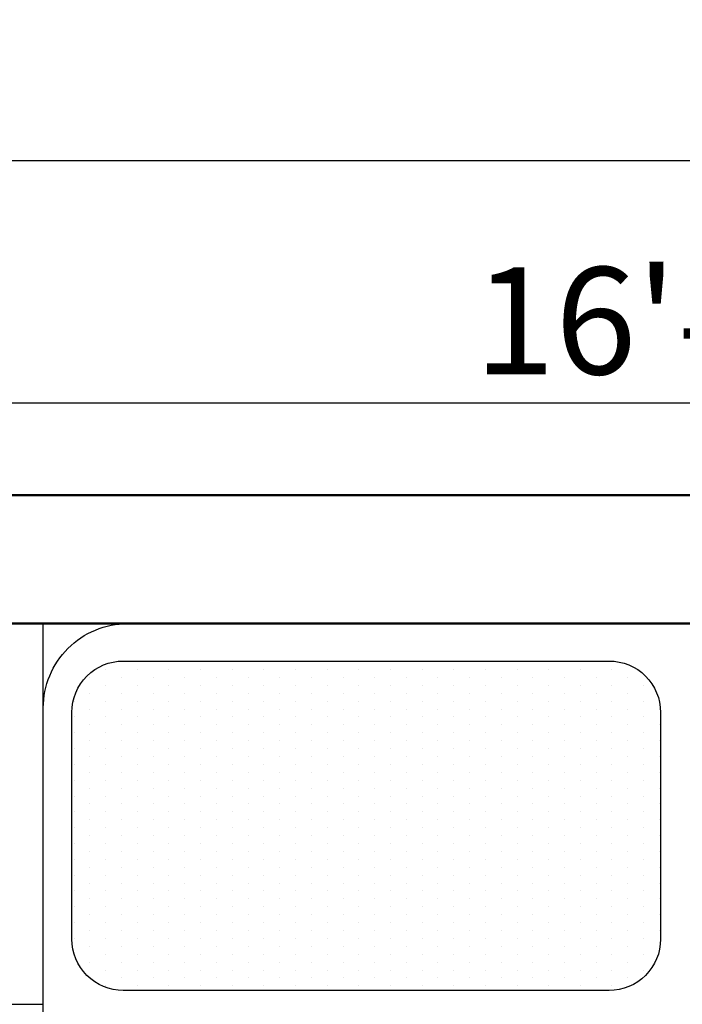
# Model space of a CAD drawing. Units: inches. Extents: x 3064 to 19385, y 846 to 15425.
# Tile 77 of 108: x 6677 to 6708, y 1964 to 2010. Entities that reach past the tile are written whole.
import ezdxf

# ---------------------------------------------------------------- set-up
doc = ezdxf.new("R2010")
doc.units = ezdxf.units.IN
for name, color, linetype, lineweight in [('A-ANNO-DIMS', 2, 'Continuous', 18), ('A-FLOR-FIXT', 9, 'Continuous', 18), ('A-WALL', 7, 'Continuous', 50)]:
    doc.layers.add(name, color=color, linetype=linetype, lineweight=lineweight)
doc.layers.add('BLOCK', color=6, linetype='Continuous')
doc.styles.get("Standard").update_dxf_attribs({"font": 'arial.ttf'})
doc.dimstyles.new('ISO-25', dxfattribs={"dimtxt": 9, "dimasz": 2.5, "dimexe": 1.25, "dimexo": 0.625, "dimtad": 1, "dimdec": 1, "dimlunit": 3, "dimtxsty": 'Standard', "dimcen": 2.5, "dimadec": 0, "dimazin": 0, "dimtfac": 1, "dimtdec": 1, "dimtmove": 0, "dimatfit": 3, "dimfxl": 1, "dimarcsym": 0})

# ---------------------------------------------------------------- blocks, each defined once
blk = doc.blocks.new('*X7')
at = {"color": 0}
for p, q in [((266.4375, 457.03125), (266.4375, 457.03125)), ((266.8125, 457.03125), (266.8125, 457.03125)), ((267.1875, 457.03125), (267.1875, 457.03125)), ((267.5625, 457.03125), (267.5625, 457.03125)), ((267.9375, 457.03125), (267.9375, 457.03125)), ((268.3125, 457.03125), (268.3125, 457.03125)), ((268.6875, 457.03125), (268.6875, 457.03125)), ((269.0625, 457.03125), (269.0625, 457.03125)), ((269.4375, 457.03125), (269.4375, 457.03125)), ((269.8125, 457.03125), (269.8125, 457.03125)), ((270.1875, 457.03125), (270.1875, 457.03125)), ((270.5625, 457.03125), (270.5625, 457.03125)), ((270.9375, 457.03125), (270.9375, 457.03125)), ((271.3125, 457.03125), (271.3125, 457.03125)), ((271.6875, 457.03125), (271.6875, 457.03125)), ((272.0625, 457.03125), (272.0625, 457.03125)), ((266.25, 456.9375), (266.25, 456.9375)), ((266.625, 456.9375), (266.625, 456.9375)), ((267, 456.9375), (267, 456.9375)), ((267.375, 456.9375), (267.375, 456.9375)), ((267.75, 456.9375), (267.75, 456.9375)), ((268.125, 456.9375), (268.125, 456.9375)), ((268.5, 456.9375), (268.5, 456.9375)), ((268.875, 456.9375), (268.875, 456.9375)), ((269.25, 456.9375), (269.25, 456.9375)), ((269.625, 456.9375), (269.625, 456.9375)), ((270, 456.9375), (270, 456.9375)), ((270.375, 456.9375), (270.375, 456.9375)), ((270.75, 456.9375), (270.75, 456.9375)), ((271.125, 456.9375), (271.125, 456.9375)), ((271.5, 456.9375), (271.5, 456.9375)), ((271.875, 456.9375), (271.875, 456.9375)), ((272.25, 456.9375), (272.25, 456.9375)), ((266.0625, 456.84375), (266.0625, 456.84375)), ((266.25, 456.75), (266.25, 456.75)), ((266.4375, 456.84375), (266.4375, 456.84375)), ((266.625, 456.75), (266.625, 456.75)), ((266.8125, 456.84375), (266.8125, 456.84375)), ((267, 456.75), (267, 456.75)), ((267.1875, 456.84375), (267.1875, 456.84375)), ((267.375, 456.75), (267.375, 456.75)), ((267.5625, 456.84375), (267.5625, 456.84375)), ((267.75, 456.75), (267.75, 456.75)), ((267.9375, 456.84375), (267.9375, 456.84375)), ((268.125, 456.75), (268.125, 456.75)), ((268.3125, 456.84375), (268.3125, 456.84375)), ((268.5, 456.75), (268.5, 456.75)), ((268.6875, 456.84375), (268.6875, 456.84375)), ((268.875, 456.75), (268.875, 456.75)), ((269.0625, 456.84375), (269.0625, 456.84375)), ((269.25, 456.75), (269.25, 456.75)), ((269.4375, 456.84375), (269.4375, 456.84375)), ((269.625, 456.75), (269.625, 456.75)), ((269.8125, 456.84375), (269.8125, 456.84375)), ((270, 456.75), (270, 456.75)), ((270.1875, 456.84375), (270.1875, 456.84375)), ((270.375, 456.75), (270.375, 456.75)), ((270.5625, 456.84375), (270.5625, 456.84375)), ((270.75, 456.75), (270.75, 456.75)), ((270.9375, 456.84375), (270.9375, 456.84375)), ((271.125, 456.75), (271.125, 456.75)), ((271.3125, 456.84375), (271.3125, 456.84375)), ((271.5, 456.75), (271.5, 456.75)), ((271.6875, 456.84375), (271.6875, 456.84375)), ((271.875, 456.75), (271.875, 456.75)), ((272.0625, 456.84375), (272.0625, 456.84375)), ((272.25, 456.75), (272.25, 456.75)), ((272.4375, 456.84375), (272.4375, 456.84375)), ((272.625, 456.75), (272.625, 456.75)), ((266.0625, 456.65625), (266.0625, 456.65625)), ((266.4375, 456.65625), (266.4375, 456.65625)), ((266.8125, 456.65625), (266.8125, 456.65625)), ((267.1875, 456.65625), (267.1875, 456.65625)), ((267.5625, 456.65625), (267.5625, 456.65625)), ((267.9375, 456.65625), (267.9375, 456.65625)), ((268.3125, 456.65625), (268.3125, 456.65625)), ((268.6875, 456.65625), (268.6875, 456.65625)), ((269.0625, 456.65625), (269.0625, 456.65625)), ((269.4375, 456.65625), (269.4375, 456.65625)), ((269.8125, 456.65625), (269.8125, 456.65625)), ((270.1875, 456.65625), (270.1875, 456.65625)), ((270.5625, 456.65625), (270.5625, 456.65625)), ((270.9375, 456.65625), (270.9375, 456.65625)), ((271.3125, 456.65625), (271.3125, 456.65625)), ((271.6875, 456.65625), (271.6875, 456.65625)), ((272.0625, 456.65625), (272.0625, 456.65625)), ((272.4375, 456.65625), (272.4375, 456.65625)), ((265.875, 456.5625), (265.875, 456.5625)), ((266.25, 456.5625), (266.25, 456.5625)), ((266.625, 456.5625), (266.625, 456.5625)), ((267, 456.5625), (267, 456.5625)), ((267.375, 456.5625), (267.375, 456.5625)), ((267.75, 456.5625), (267.75, 456.5625)), ((268.125, 456.5625), (268.125, 456.5625)), ((268.5, 456.5625), (268.5, 456.5625)), ((268.875, 456.5625), (268.875, 456.5625)), ((269.25, 456.5625), (269.25, 456.5625)), ((269.625, 456.5625), (269.625, 456.5625)), ((270, 456.5625), (270, 456.5625)), ((270.375, 456.5625), (270.375, 456.5625)), ((270.75, 456.5625), (270.75, 456.5625)), ((271.125, 456.5625), (271.125, 456.5625)), ((271.5, 456.5625), (271.5, 456.5625)), ((271.875, 456.5625), (271.875, 456.5625)), ((272.25, 456.5625), (272.25, 456.5625)), ((272.625, 456.5625), (272.625, 456.5625)), ((266.0625, 456.46875), (266.0625, 456.46875)), ((266.4375, 456.46875), (266.4375, 456.46875)), ((266.8125, 456.46875), (266.8125, 456.46875)), ((267.1875, 456.46875), (267.1875, 456.46875)), ((267.5625, 456.46875), (267.5625, 456.46875)), ((267.9375, 456.46875), (267.9375, 456.46875)), ((268.3125, 456.46875), (268.3125, 456.46875)), ((268.6875, 456.46875), (268.6875, 456.46875)), ((269.0625, 456.46875), (269.0625, 456.46875)), ((269.4375, 456.46875), (269.4375, 456.46875)), ((269.8125, 456.46875), (269.8125, 456.46875)), ((270.1875, 456.46875), (270.1875, 456.46875)), ((270.5625, 456.46875), (270.5625, 456.46875)), ((270.9375, 456.46875), (270.9375, 456.46875)), ((271.3125, 456.46875), (271.3125, 456.46875)), ((271.6875, 456.46875), (271.6875, 456.46875)), ((272.0625, 456.46875), (272.0625, 456.46875)), ((272.4375, 456.46875), (272.4375, 456.46875)), ((272.8125, 456.46875), (272.8125, 456.46875)), ((265.875, 456.375), (265.875, 456.375)), ((266.0625, 456.28125), (266.0625, 456.28125)), ((266.25, 456.375), (266.25, 456.375)), ((266.4375, 456.28125), (266.4375, 456.28125)), ((266.625, 456.375), (266.625, 456.375)), ((266.8125, 456.28125), (266.8125, 456.28125)), ((267, 456.375), (267, 456.375)), ((267.1875, 456.28125), (267.1875, 456.28125)), ((267.375, 456.375), (267.375, 456.375)), ((267.5625, 456.28125), (267.5625, 456.28125)), ((267.75, 456.375), (267.75, 456.375)), ((267.9375, 456.28125), (267.9375, 456.28125)), ((268.125, 456.375), (268.125, 456.375)), ((268.3125, 456.28125), (268.3125, 456.28125)), ((268.5, 456.375), (268.5, 456.375)), ((268.6875, 456.28125), (268.6875, 456.28125)), ((268.875, 456.375), (268.875, 456.375)), ((269.0625, 456.28125), (269.0625, 456.28125)), ((269.25, 456.375), (269.25, 456.375)), ((269.4375, 456.28125), (269.4375, 456.28125)), ((269.625, 456.375), (269.625, 456.375)), ((269.8125, 456.28125), (269.8125, 456.28125)), ((270, 456.375), (270, 456.375)), ((270.1875, 456.28125), (270.1875, 456.28125)), ((270.375, 456.375), (270.375, 456.375)), ((270.5625, 456.28125), (270.5625, 456.28125)), ((270.75, 456.375), (270.75, 456.375)), ((270.9375, 456.28125), (270.9375, 456.28125)), ((271.125, 456.375), (271.125, 456.375)), ((271.3125, 456.28125), (271.3125, 456.28125)), ((271.5, 456.375), (271.5, 456.375)), ((271.6875, 456.28125), (271.6875, 456.28125)), ((271.875, 456.375), (271.875, 456.375)), ((272.0625, 456.28125), (272.0625, 456.28125)), ((272.25, 456.375), (272.25, 456.375)), ((272.4375, 456.28125), (272.4375, 456.28125)), ((272.625, 456.375), (272.625, 456.375)), ((272.8125, 456.28125), (272.8125, 456.28125)), ((265.875, 456.1875), (265.875, 456.1875)), ((266.25, 456.1875), (266.25, 456.1875)), ((266.625, 456.1875), (266.625, 456.1875)), ((267, 456.1875), (267, 456.1875)), ((267.375, 456.1875), (267.375, 456.1875)), ((267.75, 456.1875), (267.75, 456.1875)), ((268.125, 456.1875), (268.125, 456.1875)), ((268.5, 456.1875), (268.5, 456.1875)), ((268.875, 456.1875), (268.875, 456.1875)), ((269.25, 456.1875), (269.25, 456.1875)), ((269.625, 456.1875), (269.625, 456.1875)), ((270, 456.1875), (270, 456.1875)), ((270.375, 456.1875), (270.375, 456.1875)), ((270.75, 456.1875), (270.75, 456.1875)), ((271.125, 456.1875), (271.125, 456.1875)), ((271.5, 456.1875), (271.5, 456.1875)), ((271.875, 456.1875), (271.875, 456.1875)), ((272.25, 456.1875), (272.25, 456.1875)), ((272.625, 456.1875), (272.625, 456.1875)), ((266.0625, 456.09375), (266.0625, 456.09375)), ((266.4375, 456.09375), (266.4375, 456.09375)), ((266.8125, 456.09375), (266.8125, 456.09375)), ((267.1875, 456.09375), (267.1875, 456.09375)), ((267.5625, 456.09375), (267.5625, 456.09375)), ((267.9375, 456.09375), (267.9375, 456.09375)), ((268.3125, 456.09375), (268.3125, 456.09375)), ((268.6875, 456.09375), (268.6875, 456.09375)), ((269.0625, 456.09375), (269.0625, 456.09375)), ((269.4375, 456.09375), (269.4375, 456.09375)), ((269.8125, 456.09375), (269.8125, 456.09375)), ((270.1875, 456.09375), (270.1875, 456.09375)), ((270.5625, 456.09375), (270.5625, 456.09375)), ((270.9375, 456.09375), (270.9375, 456.09375)), ((271.3125, 456.09375), (271.3125, 456.09375)), ((271.6875, 456.09375), (271.6875, 456.09375)), ((272.0625, 456.09375), (272.0625, 456.09375)), ((272.4375, 456.09375), (272.4375, 456.09375)), ((272.8125, 456.09375), (272.8125, 456.09375)), ((265.875, 456), (265.875, 456)), ((266.25, 456), (266.25, 456)), ((266.625, 456), (266.625, 456)), ((267, 456), (267, 456)), ((267.375, 456), (267.375, 456)), ((267.75, 456), (267.75, 456)), ((268.125, 456), (268.125, 456)), ((268.5, 456), (268.5, 456)), ((268.875, 456), (268.875, 456)), ((269.25, 456), (269.25, 456)), ((269.625, 456), (269.625, 456)), ((270, 456), (270, 456)), ((270.375, 456), (270.375, 456)), ((270.75, 456), (270.75, 456)), ((271.125, 456), (271.125, 456)), ((271.5, 456), (271.5, 456)), ((271.875, 456), (271.875, 456)), ((272.25, 456), (272.25, 456)), ((272.625, 456), (272.625, 456)), ((265.875, 455.8125), (265.875, 455.8125)), ((266.0625, 455.90625), (266.0625, 455.90625)), ((266.25, 455.8125), (266.25, 455.8125)), ((266.4375, 455.90625), (266.4375, 455.90625)), ((266.625, 455.8125), (266.625, 455.8125)), ((266.8125, 455.90625), (266.8125, 455.90625)), ((267, 455.8125), (267, 455.8125)), ((267.1875, 455.90625), (267.1875, 455.90625)), ((267.375, 455.8125), (267.375, 455.8125)), ((267.5625, 455.90625), (267.5625, 455.90625)), ((267.75, 455.8125), (267.75, 455.8125)), ((267.9375, 455.90625), (267.9375, 455.90625)), ((268.125, 455.8125), (268.125, 455.8125)), ((268.3125, 455.90625), (268.3125, 455.90625)), ((268.5, 455.8125), (268.5, 455.8125)), ((268.6875, 455.90625), (268.6875, 455.90625)), ((268.875, 455.8125), (268.875, 455.8125)), ((269.0625, 455.90625), (269.0625, 455.90625)), ((269.25, 455.8125), (269.25, 455.8125)), ((269.4375, 455.90625), (269.4375, 455.90625)), ((269.625, 455.8125), (269.625, 455.8125)), ((269.8125, 455.90625), (269.8125, 455.90625)), ((270, 455.8125), (270, 455.8125)), ((270.1875, 455.90625), (270.1875, 455.90625)), ((270.375, 455.8125), (270.375, 455.8125)), ((270.5625, 455.90625), (270.5625, 455.90625)), ((270.75, 455.8125), (270.75, 455.8125)), ((270.9375, 455.90625), (270.9375, 455.90625)), ((271.125, 455.8125), (271.125, 455.8125)), ((271.3125, 455.90625), (271.3125, 455.90625)), ((271.5, 455.8125), (271.5, 455.8125)), ((271.6875, 455.90625), (271.6875, 455.90625)), ((271.875, 455.8125), (271.875, 455.8125)), ((272.0625, 455.90625), (272.0625, 455.90625)), ((272.25, 455.8125), (272.25, 455.8125)), ((272.4375, 455.90625), (272.4375, 455.90625)), ((272.625, 455.8125), (272.625, 455.8125)), ((272.8125, 455.90625), (272.8125, 455.90625)), ((266.0625, 455.71875), (266.0625, 455.71875)), ((266.4375, 455.71875), (266.4375, 455.71875)), ((266.8125, 455.71875), (266.8125, 455.71875)), ((267.1875, 455.71875), (267.1875, 455.71875)), ((267.5625, 455.71875), (267.5625, 455.71875)), ((267.9375, 455.71875), (267.9375, 455.71875)), ((268.3125, 455.71875), (268.3125, 455.71875)), ((268.6875, 455.71875), (268.6875, 455.71875)), ((269.0625, 455.71875), (269.0625, 455.71875)), ((269.4375, 455.71875), (269.4375, 455.71875)), ((269.8125, 455.71875), (269.8125, 455.71875)), ((270.1875, 455.71875), (270.1875, 455.71875)), ((270.5625, 455.71875), (270.5625, 455.71875)), ((270.9375, 455.71875), (270.9375, 455.71875)), ((271.3125, 455.71875), (271.3125, 455.71875)), ((271.6875, 455.71875), (271.6875, 455.71875)), ((272.0625, 455.71875), (272.0625, 455.71875)), ((272.4375, 455.71875), (272.4375, 455.71875)), ((272.8125, 455.71875), (272.8125, 455.71875)), ((265.875, 455.625), (265.875, 455.625)), ((266.25, 455.625), (266.25, 455.625)), ((266.625, 455.625), (266.625, 455.625)), ((267, 455.625), (267, 455.625)), ((267.375, 455.625), (267.375, 455.625)), ((267.75, 455.625), (267.75, 455.625)), ((268.125, 455.625), (268.125, 455.625)), ((268.5, 455.625), (268.5, 455.625)), ((268.875, 455.625), (268.875, 455.625)), ((269.25, 455.625), (269.25, 455.625)), ((269.625, 455.625), (269.625, 455.625)), ((270, 455.625), (270, 455.625)), ((270.375, 455.625), (270.375, 455.625)), ((270.75, 455.625), (270.75, 455.625)), ((271.125, 455.625), (271.125, 455.625)), ((271.5, 455.625), (271.5, 455.625)), ((271.875, 455.625), (271.875, 455.625)), ((272.25, 455.625), (272.25, 455.625)), ((272.625, 455.625), (272.625, 455.625)), ((266.0625, 455.53125), (266.0625, 455.53125)), ((266.4375, 455.53125), (266.4375, 455.53125)), ((266.8125, 455.53125), (266.8125, 455.53125)), ((267.1875, 455.53125), (267.1875, 455.53125)), ((267.5625, 455.53125), (267.5625, 455.53125)), ((267.9375, 455.53125), (267.9375, 455.53125)), ((268.3125, 455.53125), (268.3125, 455.53125)), ((268.6875, 455.53125), (268.6875, 455.53125)), ((269.0625, 455.53125), (269.0625, 455.53125)), ((269.4375, 455.53125), (269.4375, 455.53125)), ((269.8125, 455.53125), (269.8125, 455.53125)), ((270.1875, 455.53125), (270.1875, 455.53125)), ((270.5625, 455.53125), (270.5625, 455.53125)), ((270.9375, 455.53125), (270.9375, 455.53125)), ((271.3125, 455.53125), (271.3125, 455.53125)), ((271.6875, 455.53125), (271.6875, 455.53125)), ((272.0625, 455.53125), (272.0625, 455.53125)), ((272.4375, 455.53125), (272.4375, 455.53125)), ((272.8125, 455.53125), (272.8125, 455.53125)), ((265.875, 455.4375), (265.875, 455.4375)), ((266.0625, 455.34375), (266.0625, 455.34375)), ((266.25, 455.4375), (266.25, 455.4375)), ((266.4375, 455.34375), (266.4375, 455.34375)), ((266.625, 455.4375), (266.625, 455.4375)), ((266.8125, 455.34375), (266.8125, 455.34375)), ((267, 455.4375), (267, 455.4375)), ((267.1875, 455.34375), (267.1875, 455.34375)), ((267.375, 455.4375), (267.375, 455.4375)), ((267.5625, 455.34375), (267.5625, 455.34375)), ((267.75, 455.4375), (267.75, 455.4375)), ((267.9375, 455.34375), (267.9375, 455.34375)), ((268.125, 455.4375), (268.125, 455.4375)), ((268.3125, 455.34375), (268.3125, 455.34375)), ((268.5, 455.4375), (268.5, 455.4375)), ((268.6875, 455.34375), (268.6875, 455.34375)), ((268.875, 455.4375), (268.875, 455.4375)), ((269.0625, 455.34375), (269.0625, 455.34375)), ((269.25, 455.4375), (269.25, 455.4375)), ((269.4375, 455.34375), (269.4375, 455.34375)), ((269.625, 455.4375), (269.625, 455.4375)), ((269.8125, 455.34375), (269.8125, 455.34375)), ((270, 455.4375), (270, 455.4375)), ((270.1875, 455.34375), (270.1875, 455.34375)), ((270.375, 455.4375), (270.375, 455.4375)), ((270.5625, 455.34375), (270.5625, 455.34375)), ((270.75, 455.4375), (270.75, 455.4375)), ((270.9375, 455.34375), (270.9375, 455.34375)), ((271.125, 455.4375), (271.125, 455.4375)), ((271.3125, 455.34375), (271.3125, 455.34375)), ((271.5, 455.4375), (271.5, 455.4375)), ((271.6875, 455.34375), (271.6875, 455.34375)), ((271.875, 455.4375), (271.875, 455.4375)), ((272.0625, 455.34375), (272.0625, 455.34375)), ((272.25, 455.4375), (272.25, 455.4375)), ((272.4375, 455.34375), (272.4375, 455.34375)), ((272.625, 455.4375), (272.625, 455.4375)), ((272.8125, 455.34375), (272.8125, 455.34375)), ((265.875, 455.25), (265.875, 455.25)), ((266.25, 455.25), (266.25, 455.25)), ((266.625, 455.25), (266.625, 455.25)), ((267, 455.25), (267, 455.25)), ((267.375, 455.25), (267.375, 455.25)), ((267.75, 455.25), (267.75, 455.25)), ((268.125, 455.25), (268.125, 455.25)), ((268.5, 455.25), (268.5, 455.25)), ((268.875, 455.25), (268.875, 455.25)), ((269.25, 455.25), (269.25, 455.25)), ((269.625, 455.25), (269.625, 455.25)), ((270, 455.25), (270, 455.25)), ((270.375, 455.25), (270.375, 455.25)), ((270.75, 455.25), (270.75, 455.25)), ((271.125, 455.25), (271.125, 455.25)), ((271.5, 455.25), (271.5, 455.25)), ((271.875, 455.25), (271.875, 455.25)), ((272.25, 455.25), (272.25, 455.25)), ((272.625, 455.25), (272.625, 455.25)), ((266.0625, 455.15625), (266.0625, 455.15625)), ((266.4375, 455.15625), (266.4375, 455.15625)), ((266.8125, 455.15625), (266.8125, 455.15625)), ((267.1875, 455.15625), (267.1875, 455.15625)), ((267.5625, 455.15625), (267.5625, 455.15625)), ((267.9375, 455.15625), (267.9375, 455.15625)), ((268.3125, 455.15625), (268.3125, 455.15625)), ((268.6875, 455.15625), (268.6875, 455.15625)), ((269.0625, 455.15625), (269.0625, 455.15625)), ((269.4375, 455.15625), (269.4375, 455.15625)), ((269.8125, 455.15625), (269.8125, 455.15625)), ((270.1875, 455.15625), (270.1875, 455.15625)), ((270.5625, 455.15625), (270.5625, 455.15625)), ((270.9375, 455.15625), (270.9375, 455.15625)), ((271.3125, 455.15625), (271.3125, 455.15625)), ((271.6875, 455.15625), (271.6875, 455.15625)), ((272.0625, 455.15625), (272.0625, 455.15625)), ((272.4375, 455.15625), (272.4375, 455.15625)), ((272.8125, 455.15625), (272.8125, 455.15625)), ((265.875, 455.0625), (265.875, 455.0625)), ((266.25, 455.0625), (266.25, 455.0625)), ((266.625, 455.0625), (266.625, 455.0625)), ((267, 455.0625), (267, 455.0625)), ((267.375, 455.0625), (267.375, 455.0625)), ((267.75, 455.0625), (267.75, 455.0625)), ((268.125, 455.0625), (268.125, 455.0625)), ((268.5, 455.0625), (268.5, 455.0625)), ((268.875, 455.0625), (268.875, 455.0625)), ((269.25, 455.0625), (269.25, 455.0625)), ((269.625, 455.0625), (269.625, 455.0625)), ((270, 455.0625), (270, 455.0625)), ((270.375, 455.0625), (270.375, 455.0625)), ((270.75, 455.0625), (270.75, 455.0625)), ((271.125, 455.0625), (271.125, 455.0625)), ((271.5, 455.0625), (271.5, 455.0625)), ((271.875, 455.0625), (271.875, 455.0625)), ((272.25, 455.0625), (272.25, 455.0625)), ((272.625, 455.0625), (272.625, 455.0625)), ((265.875, 454.875), (265.875, 454.875)), ((266.0625, 454.96875), (266.0625, 454.96875)), ((266.25, 454.875), (266.25, 454.875)), ((266.4375, 454.96875), (266.4375, 454.96875)), ((266.625, 454.875), (266.625, 454.875)), ((266.8125, 454.96875), (266.8125, 454.96875)), ((267, 454.875), (267, 454.875)), ((267.1875, 454.96875), (267.1875, 454.96875)), ((267.375, 454.875), (267.375, 454.875)), ((267.5625, 454.96875), (267.5625, 454.96875)), ((267.75, 454.875), (267.75, 454.875)), ((267.9375, 454.96875), (267.9375, 454.96875)), ((268.125, 454.875), (268.125, 454.875)), ((268.3125, 454.96875), (268.3125, 454.96875)), ((268.5, 454.875), (268.5, 454.875)), ((268.6875, 454.96875), (268.6875, 454.96875)), ((268.875, 454.875), (268.875, 454.875)), ((269.0625, 454.96875), (269.0625, 454.96875)), ((269.25, 454.875), (269.25, 454.875)), ((269.4375, 454.96875), (269.4375, 454.96875)), ((269.625, 454.875), (269.625, 454.875)), ((269.8125, 454.96875), (269.8125, 454.96875)), ((270, 454.875), (270, 454.875)), ((270.1875, 454.96875), (270.1875, 454.96875)), ((270.375, 454.875), (270.375, 454.875)), ((270.5625, 454.96875), (270.5625, 454.96875)), ((270.75, 454.875), (270.75, 454.875)), ((270.9375, 454.96875), (270.9375, 454.96875)), ((271.125, 454.875), (271.125, 454.875)), ((271.3125, 454.96875), (271.3125, 454.96875)), ((271.5, 454.875), (271.5, 454.875)), ((271.6875, 454.96875), (271.6875, 454.96875)), ((271.875, 454.875), (271.875, 454.875)), ((272.0625, 454.96875), (272.0625, 454.96875)), ((272.25, 454.875), (272.25, 454.875)), ((272.4375, 454.96875), (272.4375, 454.96875)), ((272.625, 454.875), (272.625, 454.875)), ((272.8125, 454.96875), (272.8125, 454.96875)), ((266.0625, 454.78125), (266.0625, 454.78125)), ((266.4375, 454.78125), (266.4375, 454.78125)), ((266.8125, 454.78125), (266.8125, 454.78125)), ((267.1875, 454.78125), (267.1875, 454.78125)), ((267.5625, 454.78125), (267.5625, 454.78125)), ((267.9375, 454.78125), (267.9375, 454.78125)), ((268.3125, 454.78125), (268.3125, 454.78125)), ((268.6875, 454.78125), (268.6875, 454.78125)), ((269.0625, 454.78125), (269.0625, 454.78125)), ((269.4375, 454.78125), (269.4375, 454.78125)), ((269.8125, 454.78125), (269.8125, 454.78125)), ((270.1875, 454.78125), (270.1875, 454.78125)), ((270.5625, 454.78125), (270.5625, 454.78125)), ((270.9375, 454.78125), (270.9375, 454.78125)), ((271.3125, 454.78125), (271.3125, 454.78125)), ((271.6875, 454.78125), (271.6875, 454.78125)), ((272.0625, 454.78125), (272.0625, 454.78125)), ((272.4375, 454.78125), (272.4375, 454.78125)), ((272.8125, 454.78125), (272.8125, 454.78125)), ((265.875, 454.6875), (265.875, 454.6875)), ((266.25, 454.6875), (266.25, 454.6875)), ((266.625, 454.6875), (266.625, 454.6875)), ((267, 454.6875), (267, 454.6875)), ((267.375, 454.6875), (267.375, 454.6875)), ((267.75, 454.6875), (267.75, 454.6875)), ((268.125, 454.6875), (268.125, 454.6875)), ((268.5, 454.6875), (268.5, 454.6875)), ((268.875, 454.6875), (268.875, 454.6875)), ((269.25, 454.6875), (269.25, 454.6875)), ((269.625, 454.6875), (269.625, 454.6875)), ((270, 454.6875), (270, 454.6875)), ((270.375, 454.6875), (270.375, 454.6875)), ((270.75, 454.6875), (270.75, 454.6875)), ((271.125, 454.6875), (271.125, 454.6875)), ((271.5, 454.6875), (271.5, 454.6875)), ((271.875, 454.6875), (271.875, 454.6875)), ((272.25, 454.6875), (272.25, 454.6875)), ((272.625, 454.6875), (272.625, 454.6875)), ((266.0625, 454.59375), (266.0625, 454.59375)), ((266.4375, 454.59375), (266.4375, 454.59375)), ((266.8125, 454.59375), (266.8125, 454.59375)), ((267.1875, 454.59375), (267.1875, 454.59375)), ((267.5625, 454.59375), (267.5625, 454.59375)), ((267.9375, 454.59375), (267.9375, 454.59375)), ((268.3125, 454.59375), (268.3125, 454.59375)), ((268.6875, 454.59375), (268.6875, 454.59375)), ((269.0625, 454.59375), (269.0625, 454.59375)), ((269.4375, 454.59375), (269.4375, 454.59375)), ((269.8125, 454.59375), (269.8125, 454.59375)), ((270.1875, 454.59375), (270.1875, 454.59375)), ((270.5625, 454.59375), (270.5625, 454.59375)), ((270.9375, 454.59375), (270.9375, 454.59375)), ((271.3125, 454.59375), (271.3125, 454.59375)), ((271.6875, 454.59375), (271.6875, 454.59375)), ((272.0625, 454.59375), (272.0625, 454.59375)), ((272.4375, 454.59375), (272.4375, 454.59375)), ((272.8125, 454.59375), (272.8125, 454.59375)), ((265.875, 454.5), (265.875, 454.5)), ((266.0625, 454.40625), (266.0625, 454.40625)), ((266.25, 454.5), (266.25, 454.5)), ((266.4375, 454.40625), (266.4375, 454.40625)), ((266.625, 454.5), (266.625, 454.5)), ((266.8125, 454.40625), (266.8125, 454.40625)), ((267, 454.5), (267, 454.5)), ((267.1875, 454.40625), (267.1875, 454.40625)), ((267.375, 454.5), (267.375, 454.5)), ((267.5625, 454.40625), (267.5625, 454.40625)), ((267.75, 454.5), (267.75, 454.5)), ((267.9375, 454.40625), (267.9375, 454.40625)), ((268.125, 454.5), (268.125, 454.5)), ((268.3125, 454.40625), (268.3125, 454.40625)), ((268.5, 454.5), (268.5, 454.5)), ((268.6875, 454.40625), (268.6875, 454.40625)), ((268.875, 454.5), (268.875, 454.5)), ((269.0625, 454.40625), (269.0625, 454.40625)), ((269.25, 454.5), (269.25, 454.5)), ((269.4375, 454.40625), (269.4375, 454.40625)), ((269.625, 454.5), (269.625, 454.5)), ((269.8125, 454.40625), (269.8125, 454.40625)), ((270, 454.5), (270, 454.5)), ((270.1875, 454.40625), (270.1875, 454.40625)), ((270.375, 454.5), (270.375, 454.5)), ((270.5625, 454.40625), (270.5625, 454.40625)), ((270.75, 454.5), (270.75, 454.5)), ((270.9375, 454.40625), (270.9375, 454.40625)), ((271.125, 454.5), (271.125, 454.5)), ((271.3125, 454.40625), (271.3125, 454.40625)), ((271.5, 454.5), (271.5, 454.5)), ((271.6875, 454.40625), (271.6875, 454.40625)), ((271.875, 454.5), (271.875, 454.5)), ((272.0625, 454.40625), (272.0625, 454.40625)), ((272.25, 454.5), (272.25, 454.5)), ((272.4375, 454.40625), (272.4375, 454.40625)), ((272.625, 454.5), (272.625, 454.5)), ((272.8125, 454.40625), (272.8125, 454.40625)), ((265.875, 454.3125), (265.875, 454.3125)), ((266.25, 454.3125), (266.25, 454.3125)), ((266.625, 454.3125), (266.625, 454.3125)), ((267, 454.3125), (267, 454.3125)), ((267.375, 454.3125), (267.375, 454.3125)), ((267.75, 454.3125), (267.75, 454.3125)), ((268.125, 454.3125), (268.125, 454.3125)), ((268.5, 454.3125), (268.5, 454.3125)), ((268.875, 454.3125), (268.875, 454.3125)), ((269.25, 454.3125), (269.25, 454.3125)), ((269.625, 454.3125), (269.625, 454.3125)), ((270, 454.3125), (270, 454.3125)), ((270.375, 454.3125), (270.375, 454.3125)), ((270.75, 454.3125), (270.75, 454.3125)), ((271.125, 454.3125), (271.125, 454.3125)), ((271.5, 454.3125), (271.5, 454.3125)), ((271.875, 454.3125), (271.875, 454.3125)), ((272.25, 454.3125), (272.25, 454.3125)), ((272.625, 454.3125), (272.625, 454.3125)), ((266.0625, 454.21875), (266.0625, 454.21875)), ((266.4375, 454.21875), (266.4375, 454.21875)), ((266.8125, 454.21875), (266.8125, 454.21875)), ((267.1875, 454.21875), (267.1875, 454.21875)), ((267.5625, 454.21875), (267.5625, 454.21875)), ((267.9375, 454.21875), (267.9375, 454.21875)), ((268.3125, 454.21875), (268.3125, 454.21875)), ((268.6875, 454.21875), (268.6875, 454.21875)), ((269.0625, 454.21875), (269.0625, 454.21875)), ((269.4375, 454.21875), (269.4375, 454.21875)), ((269.8125, 454.21875), (269.8125, 454.21875)), ((270.1875, 454.21875), (270.1875, 454.21875)), ((270.5625, 454.21875), (270.5625, 454.21875)), ((270.9375, 454.21875), (270.9375, 454.21875)), ((271.3125, 454.21875), (271.3125, 454.21875)), ((271.6875, 454.21875), (271.6875, 454.21875)), ((272.0625, 454.21875), (272.0625, 454.21875)), ((272.4375, 454.21875), (272.4375, 454.21875)), ((272.8125, 454.21875), (272.8125, 454.21875)), ((265.875, 454.125), (265.875, 454.125)), ((266.25, 454.125), (266.25, 454.125)), ((266.625, 454.125), (266.625, 454.125)), ((267, 454.125), (267, 454.125)), ((267.375, 454.125), (267.375, 454.125)), ((267.75, 454.125), (267.75, 454.125)), ((268.125, 454.125), (268.125, 454.125)), ((268.5, 454.125), (268.5, 454.125)), ((268.875, 454.125), (268.875, 454.125)), ((269.25, 454.125), (269.25, 454.125)), ((269.625, 454.125), (269.625, 454.125)), ((270, 454.125), (270, 454.125)), ((270.375, 454.125), (270.375, 454.125)), ((270.75, 454.125), (270.75, 454.125)), ((271.125, 454.125), (271.125, 454.125)), ((271.5, 454.125), (271.5, 454.125)), ((271.875, 454.125), (271.875, 454.125)), ((272.25, 454.125), (272.25, 454.125)), ((272.625, 454.125), (272.625, 454.125)), ((265.875, 453.9375), (265.875, 453.9375)), ((266.0625, 454.03125), (266.0625, 454.03125)), ((266.25, 453.9375), (266.25, 453.9375)), ((266.4375, 454.03125), (266.4375, 454.03125)), ((266.625, 453.9375), (266.625, 453.9375)), ((266.8125, 454.03125), (266.8125, 454.03125)), ((267, 453.9375), (267, 453.9375)), ((267.1875, 454.03125), (267.1875, 454.03125)), ((267.375, 453.9375), (267.375, 453.9375)), ((267.5625, 454.03125), (267.5625, 454.03125)), ((267.75, 453.9375), (267.75, 453.9375)), ((267.9375, 454.03125), (267.9375, 454.03125)), ((268.125, 453.9375), (268.125, 453.9375)), ((268.3125, 454.03125), (268.3125, 454.03125)), ((268.5, 453.9375), (268.5, 453.9375)), ((268.6875, 454.03125), (268.6875, 454.03125)), ((268.875, 453.9375), (268.875, 453.9375)), ((269.0625, 454.03125), (269.0625, 454.03125)), ((269.25, 453.9375), (269.25, 453.9375)), ((269.4375, 454.03125), (269.4375, 454.03125)), ((269.625, 453.9375), (269.625, 453.9375)), ((269.8125, 454.03125), (269.8125, 454.03125)), ((270, 453.9375), (270, 453.9375)), ((270.1875, 454.03125), (270.1875, 454.03125)), ((270.375, 453.9375), (270.375, 453.9375)), ((270.5625, 454.03125), (270.5625, 454.03125)), ((270.75, 453.9375), (270.75, 453.9375)), ((270.9375, 454.03125), (270.9375, 454.03125)), ((271.125, 453.9375), (271.125, 453.9375)), ((271.3125, 454.03125), (271.3125, 454.03125)), ((271.5, 453.9375), (271.5, 453.9375)), ((271.6875, 454.03125), (271.6875, 454.03125)), ((271.875, 453.9375), (271.875, 453.9375)), ((272.0625, 454.03125), (272.0625, 454.03125)), ((272.25, 453.9375), (272.25, 453.9375)), ((272.4375, 454.03125), (272.4375, 454.03125)), ((272.625, 453.9375), (272.625, 453.9375)), ((272.8125, 454.03125), (272.8125, 454.03125)), ((266.0625, 453.84375), (266.0625, 453.84375)), ((266.4375, 453.84375), (266.4375, 453.84375)), ((266.8125, 453.84375), (266.8125, 453.84375)), ((267.1875, 453.84375), (267.1875, 453.84375)), ((267.5625, 453.84375), (267.5625, 453.84375)), ((267.9375, 453.84375), (267.9375, 453.84375)), ((268.3125, 453.84375), (268.3125, 453.84375)), ((268.6875, 453.84375), (268.6875, 453.84375)), ((269.0625, 453.84375), (269.0625, 453.84375)), ((269.4375, 453.84375), (269.4375, 453.84375)), ((269.8125, 453.84375), (269.8125, 453.84375)), ((270.1875, 453.84375), (270.1875, 453.84375)), ((270.5625, 453.84375), (270.5625, 453.84375)), ((270.9375, 453.84375), (270.9375, 453.84375)), ((271.3125, 453.84375), (271.3125, 453.84375)), ((271.6875, 453.84375), (271.6875, 453.84375)), ((272.0625, 453.84375), (272.0625, 453.84375)), ((272.4375, 453.84375), (272.4375, 453.84375)), ((272.8125, 453.84375), (272.8125, 453.84375)), ((265.875, 453.75), (265.875, 453.75)), ((266.25, 453.75), (266.25, 453.75)), ((266.625, 453.75), (266.625, 453.75)), ((267, 453.75), (267, 453.75)), ((267.375, 453.75), (267.375, 453.75)), ((267.75, 453.75), (267.75, 453.75)), ((268.125, 453.75), (268.125, 453.75)), ((268.5, 453.75), (268.5, 453.75)), ((268.875, 453.75), (268.875, 453.75)), ((269.25, 453.75), (269.25, 453.75)), ((269.625, 453.75), (269.625, 453.75)), ((270, 453.75), (270, 453.75)), ((270.375, 453.75), (270.375, 453.75)), ((270.75, 453.75), (270.75, 453.75)), ((271.125, 453.75), (271.125, 453.75)), ((271.5, 453.75), (271.5, 453.75)), ((271.875, 453.75), (271.875, 453.75)), ((272.25, 453.75), (272.25, 453.75)), ((272.625, 453.75), (272.625, 453.75)), ((266.0625, 453.65625), (266.0625, 453.65625)), ((266.4375, 453.65625), (266.4375, 453.65625)), ((266.8125, 453.65625), (266.8125, 453.65625)), ((267.1875, 453.65625), (267.1875, 453.65625)), ((267.5625, 453.65625), (267.5625, 453.65625)), ((267.9375, 453.65625), (267.9375, 453.65625)), ((268.3125, 453.65625), (268.3125, 453.65625)), ((268.6875, 453.65625), (268.6875, 453.65625)), ((269.0625, 453.65625), (269.0625, 453.65625)), ((269.4375, 453.65625), (269.4375, 453.65625)), ((269.8125, 453.65625), (269.8125, 453.65625)), ((270.1875, 453.65625), (270.1875, 453.65625)), ((270.5625, 453.65625), (270.5625, 453.65625)), ((270.9375, 453.65625), (270.9375, 453.65625)), ((271.3125, 453.65625), (271.3125, 453.65625)), ((271.6875, 453.65625), (271.6875, 453.65625)), ((272.0625, 453.65625), (272.0625, 453.65625)), ((272.4375, 453.65625), (272.4375, 453.65625)), ((272.8125, 453.65625), (272.8125, 453.65625)), ((266.0625, 453.46875), (266.0625, 453.46875)), ((266.25, 453.5625), (266.25, 453.5625)), ((266.4375, 453.46875), (266.4375, 453.46875)), ((266.625, 453.5625), (266.625, 453.5625)), ((266.8125, 453.46875), (266.8125, 453.46875)), ((267, 453.5625), (267, 453.5625)), ((267.1875, 453.46875), (267.1875, 453.46875)), ((267.375, 453.5625), (267.375, 453.5625)), ((267.5625, 453.46875), (267.5625, 453.46875)), ((267.75, 453.5625), (267.75, 453.5625)), ((267.9375, 453.46875), (267.9375, 453.46875)), ((268.125, 453.5625), (268.125, 453.5625)), ((268.3125, 453.46875), (268.3125, 453.46875)), ((268.5, 453.5625), (268.5, 453.5625)), ((268.6875, 453.46875), (268.6875, 453.46875)), ((268.875, 453.5625), (268.875, 453.5625)), ((269.0625, 453.46875), (269.0625, 453.46875)), ((269.25, 453.5625), (269.25, 453.5625)), ((269.4375, 453.46875), (269.4375, 453.46875)), ((269.625, 453.5625), (269.625, 453.5625)), ((269.8125, 453.46875), (269.8125, 453.46875)), ((270, 453.5625), (270, 453.5625)), ((270.1875, 453.46875), (270.1875, 453.46875)), ((270.375, 453.5625), (270.375, 453.5625)), ((270.5625, 453.46875), (270.5625, 453.46875)), ((270.75, 453.5625), (270.75, 453.5625)), ((270.9375, 453.46875), (270.9375, 453.46875)), ((271.125, 453.5625), (271.125, 453.5625)), ((271.3125, 453.46875), (271.3125, 453.46875)), ((271.5, 453.5625), (271.5, 453.5625)), ((271.6875, 453.46875), (271.6875, 453.46875)), ((271.875, 453.5625), (271.875, 453.5625)), ((272.0625, 453.46875), (272.0625, 453.46875)), ((272.25, 453.5625), (272.25, 453.5625)), ((272.4375, 453.46875), (272.4375, 453.46875)), ((272.625, 453.5625), (272.625, 453.5625)), ((266.25, 453.375), (266.25, 453.375)), ((266.625, 453.375), (266.625, 453.375)), ((267, 453.375), (267, 453.375)), ((267.375, 453.375), (267.375, 453.375)), ((267.75, 453.375), (267.75, 453.375)), ((268.125, 453.375), (268.125, 453.375)), ((268.5, 453.375), (268.5, 453.375)), ((268.875, 453.375), (268.875, 453.375)), ((269.25, 453.375), (269.25, 453.375)), ((269.625, 453.375), (269.625, 453.375)), ((270, 453.375), (270, 453.375)), ((270.375, 453.375), (270.375, 453.375)), ((270.75, 453.375), (270.75, 453.375)), ((271.125, 453.375), (271.125, 453.375)), ((271.5, 453.375), (271.5, 453.375)), ((271.875, 453.375), (271.875, 453.375)), ((272.25, 453.375), (272.25, 453.375)), ((272.625, 453.375), (272.625, 453.375)), ((266.0625, 453.28125), (266.0625, 453.28125)), ((266.4375, 453.28125), (266.4375, 453.28125)), ((266.8125, 453.28125), (266.8125, 453.28125)), ((267.1875, 453.28125), (267.1875, 453.28125)), ((267.5625, 453.28125), (267.5625, 453.28125)), ((267.9375, 453.28125), (267.9375, 453.28125)), ((268.3125, 453.28125), (268.3125, 453.28125)), ((268.6875, 453.28125), (268.6875, 453.28125)), ((269.0625, 453.28125), (269.0625, 453.28125)), ((269.4375, 453.28125), (269.4375, 453.28125)), ((269.8125, 453.28125), (269.8125, 453.28125)), ((270.1875, 453.28125), (270.1875, 453.28125)), ((270.5625, 453.28125), (270.5625, 453.28125)), ((270.9375, 453.28125), (270.9375, 453.28125)), ((271.3125, 453.28125), (271.3125, 453.28125)), ((271.6875, 453.28125), (271.6875, 453.28125)), ((272.0625, 453.28125), (272.0625, 453.28125)), ((272.4375, 453.28125), (272.4375, 453.28125)), ((266.25, 453.1875), (266.25, 453.1875)), ((266.625, 453.1875), (266.625, 453.1875)), ((267, 453.1875), (267, 453.1875)), ((267.375, 453.1875), (267.375, 453.1875)), ((267.75, 453.1875), (267.75, 453.1875)), ((268.125, 453.1875), (268.125, 453.1875)), ((268.5, 453.1875), (268.5, 453.1875)), ((268.875, 453.1875), (268.875, 453.1875)), ((269.25, 453.1875), (269.25, 453.1875)), ((269.625, 453.1875), (269.625, 453.1875)), ((270, 453.1875), (270, 453.1875)), ((270.375, 453.1875), (270.375, 453.1875)), ((270.75, 453.1875), (270.75, 453.1875)), ((271.125, 453.1875), (271.125, 453.1875)), ((271.5, 453.1875), (271.5, 453.1875)), ((271.875, 453.1875), (271.875, 453.1875)), ((272.25, 453.1875), (272.25, 453.1875))]:
    blk.add_line(p, q, dxfattribs=at)
blk = doc.blocks.new('A$C52E67D0D')
at = {"layer": 'BLOCK'}
blk.add_lwpolyline([(501, 1348.6), (501, 1799.6), (0, 1799.6), (0, 1348.6)], close=True, dxfattribs=at)
for points in [[(1901, 0), (601, 0, -0.414214), (501, 100), (501, 1700, -0.414214), (601, 1800), (1901, 1800, -0.414214), (2001, 1700), (2001, 100, -0.414214)], [(1171.8, 1365.1), (595.8, 1365.1, -0.414214), (535, 1425.9), (535, 1694.8, -0.414214), (595.8, 1755.7), (1171.8, 1755.7, -0.414214), (1232.6, 1694.8), (1232.6, 1425.9, -0.414214)]]:
    blk.add_lwpolyline(points, format="xyb", close=True, dxfattribs=at)
blk.add_arc((1888.6, -1664.5), 3015.3, 87.8642, 117.4001, dxfattribs=at)
at = {"layer": 'BLOCK', "xscale": 100, "yscale": 100, "zscale": 100}
blk.add_blockref('*X7', (-26050, -43948.2), dxfattribs=at)
blk = doc.blocks.new('*D344')
at = {"layer": 'A-ANNO-DIMS', "color": 0, "lineweight": -2, "transparency": 16777216}
for p, q in [((6610.034, 1988.614), (6610.034, 1993.551)), ((6805.034, 1988.614), (6805.034, 1993.551)), ((6612.534, 1992.301), (6802.534, 1992.301))]:
    blk.add_line(p, q, dxfattribs=at)
at = {"layer": 'A-ANNO-DIMS', "color": 0, "transparency": 16777216}
for points in [[(6612.534, 1992.718), (6612.534, 1991.884), (6610.034, 1992.301)], [(6802.534, 1992.718), (6802.534, 1991.884), (6805.034, 1992.301)]]:
    blk.add_solid(points, dxfattribs=at)
at = {"layer": 'Defpoints', "color": 0, "transparency": 16777216}
for p in [(6805.034, 1992.301), (6610.034, 1987.989), (6805.034, 1987.989)]:
    blk.add_point(p, dxfattribs=at)
at = {"layer": 'A-ANNO-DIMS', "color": 0, "transparency": 16777216, "insert": (6707.534, 1995.481), "char_height": 5, "attachment_point": 5}
blk.add_mtext('16\'-3"', dxfattribs=at)
blk = doc.blocks.new('*D340')
at = {"layer": 'A-ANNO-DIMS', "color": 0, "lineweight": -2, "transparency": 16777216}
for p, q in [((6469.034, 1988.614), (6469.034, 2004.848)), ((6811.034, 1988.614), (6811.034, 2004.848)), ((6808.534, 2003.598), (6471.534, 2003.598))]:
    blk.add_line(p, q, dxfattribs=at)
at = {"layer": 'A-ANNO-DIMS', "color": 0, "transparency": 16777216}
for points in [[(6471.534, 2004.015), (6471.534, 2003.182), (6469.034, 2003.598)], [(6808.534, 2004.015), (6808.534, 2003.182), (6811.034, 2003.598)]]:
    blk.add_solid(points, dxfattribs=at)
at = {"layer": 'Defpoints', "color": 0, "transparency": 16777216}
for p in [(6469.034, 2003.598), (6469.034, 1987.989), (6811.034, 1987.989)]:
    blk.add_point(p, dxfattribs=at)
at = {"layer": 'A-ANNO-DIMS', "color": 0, "transparency": 16777216, "insert": (6640.034, 2006.776), "char_height": 5, "attachment_point": 5}
blk.add_mtext('28\'-6"', dxfattribs=at)

msp = doc.modelspace()

# ---------------------------------------------------------------- linework, layer by layer
at = {"layer": 'A-WALL'}
for p, q in [((6811.034, 1987.989), (6469.034, 1987.989)), ((6805.034, 1981.989), (6610.034, 1981.989))]:
    msp.add_line(p, q, dxfattribs=at)

# ---------------------------------------------------------------- block references
at = {"layer": 'A-FLOR-FIXT', "xscale": 0.039370099999992, "yscale": 0.039370099999992, "zscale": 0.039370099999992}
msp.add_blockref('A$C52E67D0D', (6658.282, 1911.123), dxfattribs=at)

# ---------------------------------------------------------------- dimensions: what is measured, and where the dimension line sits
at = {"layer": 'A-ANNO-DIMS'}
for base, p1, p2, override, picture, middle in [((6469.034, 2003.598), (6811.034, 1987.989), (6469.034, 1987.989), {"dimtxt": 5, "dimclrd": 0, "dimclre": 0, "dimclrt": 0}, '*D340', (6640.034, 2006.776)), ((6805.034, 1992.301), (6610.034, 1987.989), (6805.034, 1987.989), {"dimtxt": 5, "dimclrd": 0, "dimclre": 0, "dimclrt": 0, "dimtmove": 1}, '*D344', (6707.534, 1995.481))]:
    dim = msp.add_linear_dim(base=base, p1=p1, p2=p2, dimstyle='ISO-25', override=override, dxfattribs=at)
    dim.commit()
    dim.dimension.update_dxf_attribs({"geometry": picture, "text_midpoint": middle})

doc.saveas('drawing.dxf')
